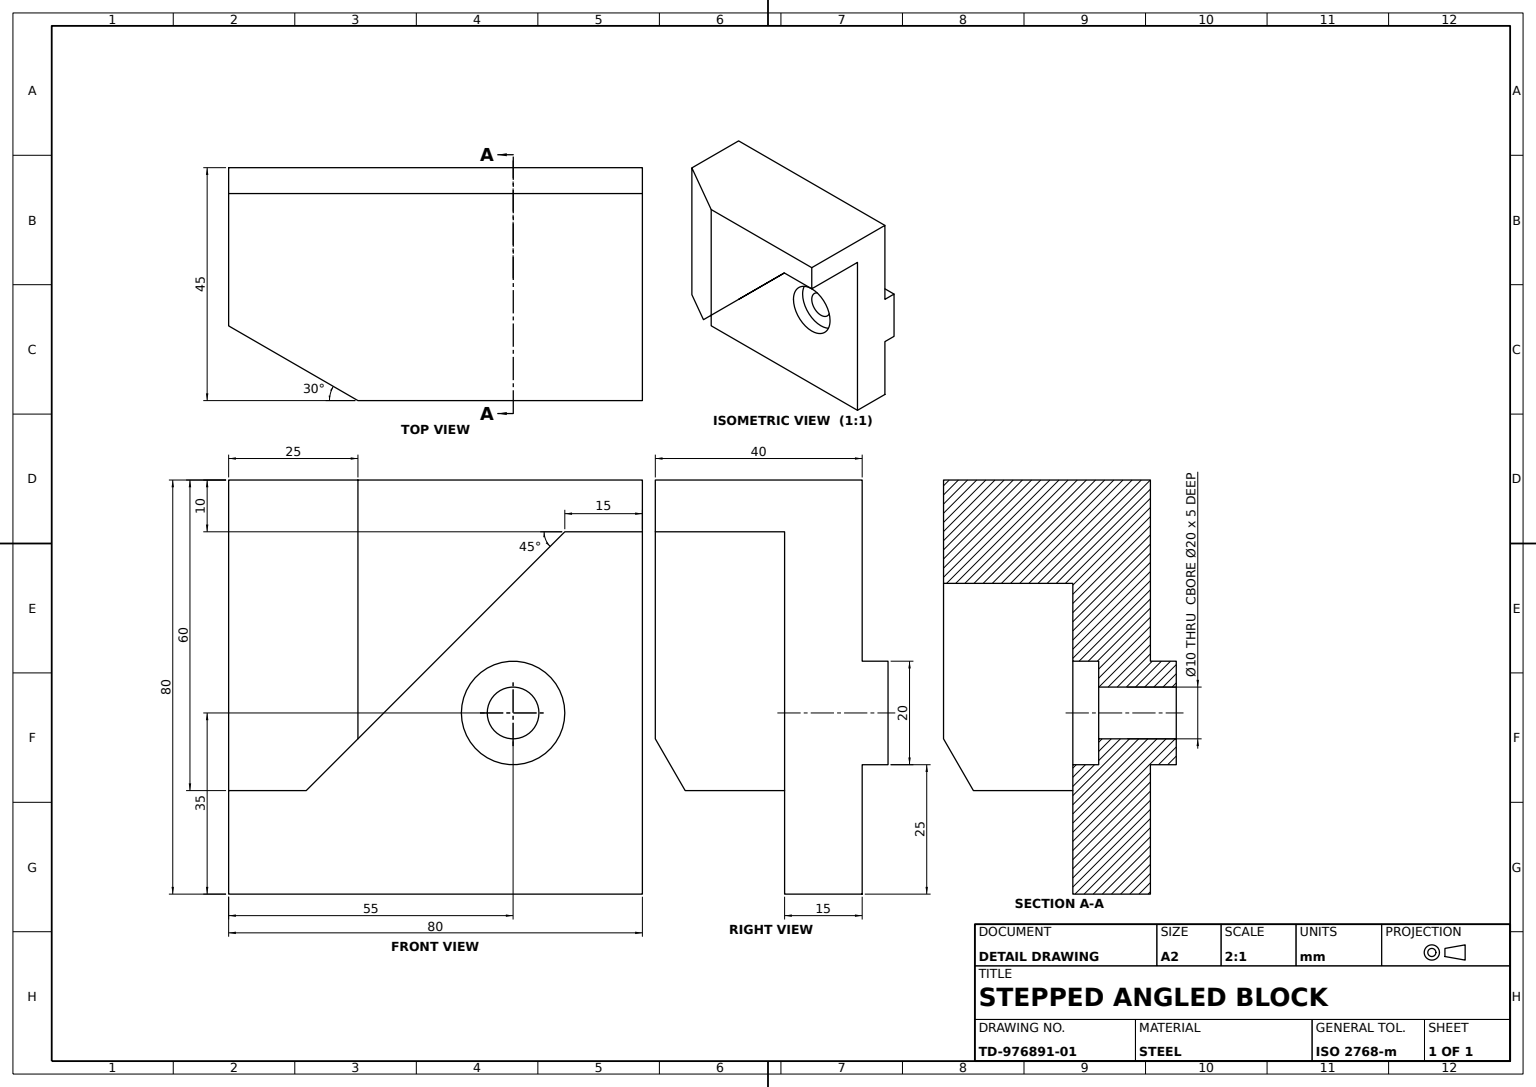
SolidWorks part; units mm, degrees
material "Plain Carbon Steel"
ref_plane "Front Plane" through (0, 0, 0) normal (0, 0, 1) x (1, 0, 0)
ref_plane "Top Plane" through (0, 0, 0) normal (0, 1, 0) x (1, 0, 0)
ref_plane "Right Plane" through (0, 0, 0) normal (1, 0, 0) x (0, 0, -1)
sketch "Base Plate Sketch" plane through (0, 0, 0) normal (0, 0, 1) x (1, 0, 0)
  line L0 (0, 0) -> (80, 0)
  line L1 (80, 0) -> (80, -80)
  line L2 (80, -80) -> (0, -80)
  line L3 (0, -80) -> (0, 0)
  dimension "D1" = 80
  dimension "D2" = 80
extrude "Base Plate 80x80x15" add sketch "Base Plate Sketch" along normal blind 15
sketch "Vertical Wall Sketch" plane through (80, 0, 0) normal (1, 0, 0) x (0, 0, -1)
  line L0 (-15, 0) -> (0, 0) construction
  line L1 (0, -80) -> (0, 0) construction
  line L2 (0, -55) -> (5, -55)
  line L3 (5, -55) -> (5, -35)
  line L4 (5, -35) -> (0, -35)
  line L5 (0, -35) -> (0, -55)
  dimension "D1" = 5
  dimension "D2" = 35
  dimension "D3" = 55
extrude "Vertical Wall" add sketch "Vertical Wall Sketch" against normal blind 80
sketch "Step Boss Sketch" plane through (0, 0, 0) normal (0, 1, 0) x (1, 0, 0)
  line L0 (0, -15) -> (0, 0) construction
  line L1 (80, -15) -> (80, -40)
  line L2 (80, -15) -> (0, -15) construction
  line L3 (25, -15) -> (25, -40)
  line L4 (25, -40) -> (80, -40)
  line L5 (80, 0) -> (0, 0) construction
  line L6 (25, -15) -> (80, -15)
  dimension "D1" = 25
  dimension "D2" = 40
extrude "Step Boss" add sketch "Step Boss Sketch" against normal blind 10
sketch "V Block Body Sketch" plane through (0, 0, 0) normal (0, 1, 0) x (1, 0, 0)
  line L0 (25, -40) -> (0, -25.5662)
  line L1 (25, -15) -> (25, -40) construction
  line L3 (0, -15) -> (0, -25.5662)
  line L4 (0, -15) -> (25, -15)
  line L5 (25, -15) -> (25, -40)
  line L7 (80, 0) -> (0, 0) construction
  dimension "D1" = 25.5662
extrude "V Block Body" add sketch "V Block Body Sketch" against normal blind 60
sketch "Angled Boss 45deg Sketch" plane through (0, 0, 40) normal (0, 0, 1) x (1, 0, 0)
  line L1 (80, -10) -> (25, -10) construction
  line L2 (65, -10) -> (31.3743, -43.6257)
  line L3 (31.3743, -43.6257) -> (25, -50)
  line L4 (25, -60) -> (25, -10) construction
  line L5 (25, -10) -> (65, -10)
  line L6 (25, -10) -> (25, -50)
  dimension "D1" = 45
  dimension "D2" = 40
  dimension "D3" = 9.0147
extrude "Angled Boss 45deg" add sketch "Angled Boss 45deg Sketch" against normal blind 25
sketch "V Groove Sketch" plane through (0, 0, 40) normal (0, 0, 1) x (1, 0, 0)
  line L0 (25, -50) -> (15, -60)
  line L1 (25, -60) -> (0, -60) construction
  line L2 (15, -60) -> (25, -60)
  line L3 (25, -60) -> (25, -50)
extrude "V Groove Cut" cut sketch "V Groove Sketch" against normal blind 25
sketch "Counterbore Sketch" plane through (0, 0, 15) normal (0, 0, 1) x (1, 0, 0)
  line L0 (80, -80) -> (55, -80)
  line L1 (0, -80) -> (80, -80) construction
  line L2 (55, -80) -> (55, -45)
  line L3 (0, -60) -> (0, -80) construction
  line L4 (15, -60) -> (0, -60) construction
  circle A0 centre (55, -45) radius 10
  dimension "D1" = 20
  dimension "D2" = 20
  dimension "D3" = 55
  dimension "D4" = 15
extrude "Counterbore Ø20x5" cut sketch "Counterbore Sketch" against normal blind 5
sketch "Hole Sketch" plane through (0, 0, 10) normal (0, 0, 1) x (1, 0, 0)
  circle A0 centre (55, -45) radius 5
  dimension "D1" = 10
  dimension "D2" = 10
extrude "Hole Ø10" cut sketch "Hole Sketch" against normal blind 20
